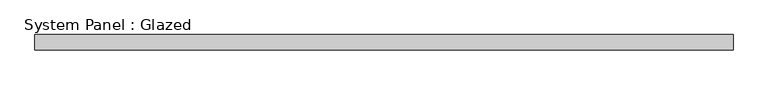
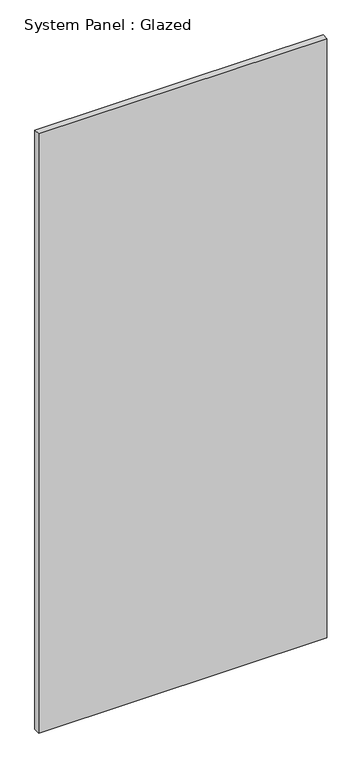
"""IFC4 building model written with IfcOpenShell, lengths in millimetres: plate geometry, System Panel : Glazed."""

from ifc_helpers import new_model, si_unit, origin, origin_with_axes, place, context, project, spatial, polyline, outline, extrude, source, transform, mapped, element, save


def system_panel_glazed_214c7444(model_context):
    return source(origin(), model_context, "Body", "SweptSolid", [
        extrude(outline(polyline([(577.85, 19.05), (-577.85, 19.05), (-577.85, 44.45), (577.85, 44.45), (577.85, 19.05)])), origin_with_axes(), (0.0, 0.0, 1.0), 2540.0),
    ])


if __name__ == "__main__":
    model = new_model("IFC4")
    model_context = context("Model", 3, world=origin())
    ifc_project = project(units=[si_unit("LENGTHUNIT", "METRE", prefix="MILLI")], contexts=[model_context])
    site = spatial("IfcSite", under=ifc_project)
    building = spatial("IfcBuilding", under=site)
    placement = place(None, origin())
    system_panel_glazed_shape = system_panel_glazed_214c7444(model_context)
    element("IfcPlate", 1, ObjectType="System Panel : Glazed", at=placement, inside=building, context=model_context, shape_type="MappedRepresentation", body=[
        mapped(system_panel_glazed_shape, transform((0.0, 0.0, 0.0), x_axis=(1.0, 0.0, 0.0), y_axis=(0.0, 1.0, 0.0), z_axis=(0.0, 0.0, 1.0))),
    ])
    save(model, "model.ifc")

# Revit data of these elements
# Type "System Panel : Glazed"
#   Construction Type Id = "GSP4R"
#   Analytic Construction = "1/8 in Pilkington single glazing"
#   Visual Light Transmittance = 0.9
#   Solar Heat Gain Coefficient = 0.86
#   Heat Transfer Coefficient (U) = 1.18115 BTU/(h·ft²·°F)
#   Define Thermal Properties by = 1
# Element 1 (IfcPlate, "System Panel : Glazed")
#   Materials on its faces: "Glass"
# Materials
#   "Glass": class "Glass", colour RGB 0 128 192, transparency 0.75, Description = "Soda Lime Glass", Cost = 0
